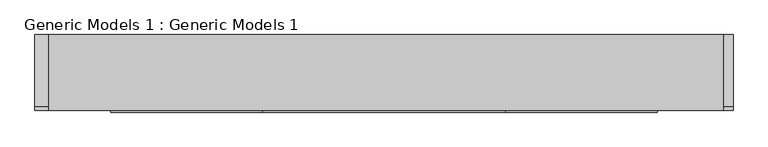
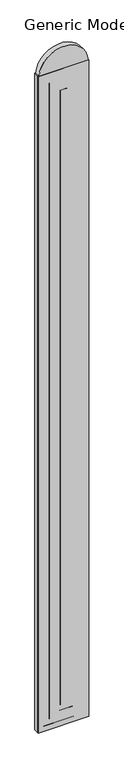
"""IFC4 building model written with IfcOpenShell, lengths in millimetres: proxy geometry, Generic Models 1 : Generic Models 1."""

from ifc_helpers import new_model, si_unit, point, frame, frame_2d, origin, origin_with_axes, place, context, project, spatial, polyline, circle_curve, trimmed, segment, composite_curve, outline, extrude, source, transform, mapped, element, save


def generic_models_1_generic_models_1_ee720f7e(model_context):
    return source(origin(), model_context, "Body", "SweptSolid", [
        extrude(outline(polyline([(1404.7271285, -6235.9544725), (-930.7154463, -6235.9544725), (-930.7154463, -6223.9490038), (1404.7271285, -6223.9490038), (1404.7271285, -6235.9544725)])), origin_with_axes(), (0.0, 0.0, 1.0), 31851.6),
        extrude(outline(polyline([(0.0, -930.7154463), (0.0, 1404.7271285), (31851.6, 1404.7271285), (31851.6, -930.7154463), (0.0, -930.7154463)]), holes=[polyline([(31597.6, 1150.7271285), (254.0, 1150.7271285), (254.0, -676.7154463), (31597.6, -676.7154463), (31597.6, 1150.7271285)])]), frame((0.0, -6235.9544725, 0.0), z_axis=(0.0, 1.0, 0.0), x_axis=(0.0, 0.0, 1.0)), (0.0, 0.0, 1.0), 254.0),
        extrude(outline(polyline([(31343.6, 896.7271285), (31343.6, -422.7154463), (508.0, -422.7154463), (508.0, 896.7271285), (31343.6, 896.7271285)]), holes=[polyline([(31089.6, 642.7271285), (762.0, 642.7271285), (762.0, -168.7154463), (31089.6, -168.7154463), (31089.6, 642.7271285)])]), frame((0.0, -6235.9544725, 0.0), z_axis=(0.0, 1.0, 0.0), x_axis=(0.0, 0.0, 1.0)), (0.0, 0.0, 1.0), 254.0),
        extrude(outline(polyline([(85.2845537, -6235.9544725), (85.2845537, -5981.9544725), (388.7271285, -5981.9544725), (388.7271285, -6235.9544725), (85.2845537, -6235.9544725)])), frame((0.0, 0.0, 1016.0), z_axis=(0.0, 0.0, 1.0), x_axis=(1.0, 0.0, 0.0)), (0.0, 0.0, 1.0), 29819.6),
        extrude(outline(composite_curve([segment(trimmed(circle_curve(frame_2d((31775.4, 243.3558411)), 1132.0178178), [point((31851.6, 1372.8061056))], [point((31851.6, -886.0944233))], False, "CARTESIAN"), True, "CONTINUOUS"), segment(polyline([(31851.6, -886.0944233), (31851.6, 1372.8061056)]), True, "CONTINUOUS")], self_intersect=False)), frame((0.0, -6235.9544725, 0.0), z_axis=(0.0, 1.0, 0.0), x_axis=(0.0, 0.0, 1.0)), (0.0, 0.0, 1.0), 254.0),
    ])


if __name__ == "__main__":
    model = new_model("IFC4")
    model_context = context("Model", 3, world=origin())
    ifc_project = project(units=[si_unit("LENGTHUNIT", "METRE", prefix="MILLI")], contexts=[model_context])
    site = spatial("IfcSite", under=ifc_project)
    building = spatial("IfcBuilding", under=site)
    placement = place(None, origin())
    generic_models_1_generic_models_1_shape = generic_models_1_generic_models_1_ee720f7e(model_context)
    element("IfcBuildingElementProxy", 1, Name="Generic Models 1 : Generic Models 1", ObjectType="Generic Models 1 : Generic Models 1", at=placement, inside=building, context=model_context, shape_type="MappedRepresentation", body=[
        mapped(generic_models_1_generic_models_1_shape, transform((0.0, 0.0, 0.0), x_axis=(1.0, 0.0, 0.0), y_axis=(0.0, 1.0, 0.0), z_axis=(0.0, 0.0, 1.0))),
    ])
    save(model, "model.ifc")

# Revit data of these elements
# Element 1 (IfcBuildingElementProxy, "Generic Models 1 : Generic Models 1")
#   Materials on its faces: "Brick, Common", "Gypsum Wall Board", "MARBLE"
# Materials
#   "Brick, Common": class "Masonry", colour RGB 170 98 104, transparency 0, Description = "Common brick", Cost = 0
#   "Gypsum Wall Board": class "Generic", colour RGB 127 127 127, transparency 0, Description = "Gypsum Wall Board", Cost = 0
#   "MARBLE": class "Generic", colour RGB 120 120 120, transparency 0, Cost = 0
